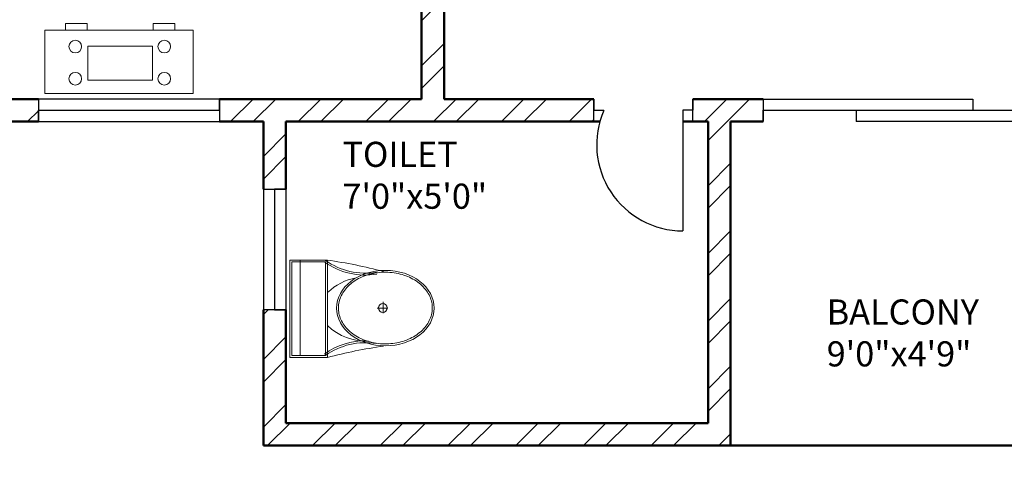
# Model space of a CAD drawing. Units: inches. Extents: x 963 to 2075, y 289 to 2657.
# Tile 45 of 98: x 1689 to 1885, y 1474 to 1563. Entities that reach past the tile are written whole.
import ezdxf

# ---------------------------------------------------------------- set-up
doc = ezdxf.new("R2010")
doc.units = ezdxf.units.IN
for name, color, linetype, lineweight in [('A-AREA-IDEN', 7, 'Continuous', 18), ('A-DOOR', 4, 'Continuous', 25), ('A-FLOR-FIXT', 9, 'Continuous', 18), ('A-GLAZ', 3, 'Continuous', 25), ('A-WALL', 7, 'Continuous', 50), ('A-WALL-PATT', 8, 'Continuous', 13)]:
    doc.layers.add(name, color=color, linetype=linetype, lineweight=lineweight)
doc.styles.get("Standard").update_dxf_attribs({"font": 'arial.ttf'})

# ---------------------------------------------------------------- blocks, each defined once
blk = doc.blocks.new('A$C31115884')
for p, q in [((283.1, 497.7), (223.4, 497.7)), ((257.5, 466.4), (257.5, 523.2)), ((0, 200), (0, 0)), ((520, 200), (0, 200)), ((10, 190), (10, 10)), ((510, 190), (10, 190)), ((510, 10), (510, 190)), ((520, 0), (520, 200)), ((510, 54.5), (0, 54.5)), ((10, 10), (510, 10)), ((0, 0), (520, 0))]:
    blk.add_line(p, q)
blk.add_circle((255.6, 496.4), 23.6)
for centre, radius, start, end in [((2777.7, -204.6), 2807, 165.4549, 171.7133), ((3237, 905), 2807, 188.2867, 194.5451), ((-294.5, 403.3), 364.7, 324.2091, 9.3499), ((-294.5, 403.3), 374.7, 324.2091, 9.3499), ((805.8, 403.3), 364.7, 170.6501, 215.7909), ((139.5, 406.2), 293.5, 315.8436, 2.6563), ((805.8, 403.3), 374.7, 179.2036, 215.7909), ((383.6, 406.2), 293.5, 190.2774, 224.1564)]:
    blk.add_arc(centre, radius, start, end)
blk.add_ellipse((256.2, 509.9), major_axis=(0, -260.7), ratio=0.772727)
blk.add_open_spline([(256.2, 259.2), (263.1, 259.2), (270, 259.7), (287.8, 262.3), (298.7, 265.1), (319.9, 273.1), (330.2, 278.4), (350.1, 291.1), (359.7, 298.7), (377.7, 315.9), (386.2, 325.5), (401.7, 346.6), (408.8, 358.1), (421.3, 382.5), (426.8, 395.5), (435.9, 422.4), (439.5, 436.4), (444.8, 465.1), (446.5, 479.7), (447.9, 509.2), (447.6, 524), (445, 553.3), (442.7, 567.8), (436.3, 596), (432.1, 609.7), (421.9, 636), (416, 648.6), (402.5, 672.1), (395, 683), (378.6, 703), (369.8, 712.1), (351.1, 728), (341.3, 734.8), (320.9, 746.2), (310.4, 750.7), (288.9, 757.3), (278, 759.4), (256, 761), (245, 760.6), (223.1, 757.2), (212.3, 754.3), (191.1, 746.1), (180.8, 740.7), (160.9, 727.8), (151.4, 720.1), (133.5, 702.7), (125.1, 693), (109.6, 671.7), (102.6, 660.2), (90.2, 635.7), (84.9, 622.7), (76, 595.6), (72.4, 581.6), (67.2, 552.9), (65.6, 538.2), (64.4, 508.8), (64.8, 494), (67.5, 464.7), (69.9, 450.2), (76.6, 422), (80.8, 408.3), (91.1, 382.2), (97.2, 369.7), (110.8, 346.3), (118.4, 335.4), (134.8, 315.6), (143.7, 306.7), (162.4, 290.9), (172.3, 284.2), (192.8, 273), (203.3, 268.6), (224.8, 262.2), (235.8, 260.2), (249.9, 259.3), (253, 259.2), (256.2, 259.2)], degree=3, knots=[0, 0, 0, 0, 0.110105, 0.110105, 0.285049, 0.285049, 0.459994, 0.459994, 0.634938, 0.634938, 0.809882, 0.809882, 0.984827, 0.984827, 1.159771, 1.159771, 1.334715, 1.334715, 1.50966, 1.50966, 1.684604, 1.684604, 1.859549, 1.859549, 2.034493, 2.034493, 2.209437, 2.209437, 2.384382, 2.384382, 2.559326, 2.559326, 2.73427, 2.73427, 2.909215, 2.909215, 3.084159, 3.084159, 3.259103, 3.259103, 3.434048, 3.434048, 3.608992, 3.608992, 3.783936, 3.783936, 3.958881, 3.958881, 4.133825, 4.133825, 4.30877, 4.30877, 4.483714, 4.483714, 4.658658, 4.658658, 4.833603, 4.833603, 5.008547, 5.008547, 5.183491, 5.183491, 5.358436, 5.358436, 5.53338, 5.53338, 5.708324, 5.708324, 5.883269, 5.883269, 6.058213, 6.058213, 6.233158, 6.233158, 6.283185, 6.283185, 6.283185, 6.283185])

msp = doc.modelspace()

# ---------------------------------------------------------------- hatches: boundary and pattern name
at = {"layer": 'A-WALL-PATT'}
h = msp.add_hatch(dxfattribs=at)
h.set_pattern_fill('ANSI32', color=256)
h.paths.add_polyline_path([(1296.92, 2558.32), (1203.92, 2558.32), (1203.92, 2493.82), (1191.53, 2493.82), (1191.53, 2489.32), (1211.06, 2489.32), (1211.06, 2492.02), (1211.06, 2493.82), (1208.42, 2493.82), (1208.42, 2553.82), (1292.42, 2553.82), (1292.42, 2538.86), (1296.92, 2538.86)])
h.paths.add_polyline_path([(1442.42, 2558.32), (1349.42, 2558.32), (1349.42, 2538.94), (1353.92, 2538.94), (1353.92, 2553.82), (1437.92, 2553.82), (1437.92, 2493.82), (1434.54, 2493.82), (1434.54, 2489.32), (1448.31, 2489.32), (1448.31, 2491.57), (1448.31, 2493.82), (1442.42, 2493.82)])
h.paths.add_polyline_path([(1415.55, 2491.57), (1415.55, 2493.82), (1340.94, 2493.82), (1340.94, 2489.32), (1371.92, 2489.32), (1371.92, 2378.32), (1367.6, 2378.32), (1367.6, 2373.82), (1371.92, 2373.82), (1371.92, 2355.19), (1376.42, 2355.19), (1376.42, 2489.32), (1415.55, 2489.32)])
h.paths.add_polyline_path([(1304.94, 2491.57), (1304.94, 2493.82), (1296.92, 2493.82), (1296.92, 2514.86), (1292.42, 2514.86), (1292.42, 2493.82), (1232.81, 2493.82), (1232.81, 2489.32), (1256.42, 2489.32), (1256.42, 2327.32), (1253.71, 2327.32), (1253.71, 2322.82), (1328.42, 2322.82), (1328.42, 2331.15), (1323.92, 2331.15), (1323.92, 2327.32), (1260.92, 2327.32), (1260.92, 2373.82), (1323.92, 2373.82), (1323.92, 2357.81), (1328.42, 2357.81), (1328.42, 2373.82), (1346.01, 2373.82), (1346.01, 2376.07), (1346.01, 2378.32), (1260.92, 2378.32), (1260.92, 2489.32), (1304.94, 2489.32)])
h.paths.add_polyline_path([(1226.65, 2327.32), (1124.42, 2327.32), (1124.42, 2347.45), (1119.92, 2347.45), (1119.92, 2322.82), (1163.42, 2322.82), (1163.42, 2305.43), (1165.67, 2305.43), (1167.92, 2305.43), (1167.92, 2322.82), (1226.65, 2322.82), (1226.65, 2325.07)])
h.paths.add_polyline_path([(1095.92, 2489.32), (1124.42, 2489.32), (1131.53, 2489.32), (1131.53, 2491.57), (1131.53, 2493.82), (1119.92, 2493.82), (1091.42, 2493.82), (1091.42, 2417.32), (1095.92, 2417.32), (1119.92, 2417.32), (1119.92, 2407.45), (1124.42, 2407.45), (1124.42, 2421.82), (1095.92, 2421.82)])
h.paths.add_polyline_path([(1512.92, 2558.32), (1508.42, 2558.32), (1508.42, 2493.82), (1503.4, 2493.82), (1503.4, 2489.32), (1508.42, 2489.32), (1508.42, 2327.32), (1376.42, 2327.32), (1376.42, 2330.27), (1371.92, 2330.27), (1371.92, 2298.74), (1376.42, 2298.74), (1376.42, 2322.82), (1508.42, 2322.82), (1508.42, 2165.32), (1504.26, 2165.32), (1504.26, 2160.82), (1508.42, 2160.82), (1508.42, 2108.32), (1512.92, 2108.32), (1512.92, 2160.82), (1516.18, 2160.82), (1516.18, 2163.07), (1516.18, 2165.32), (1512.92, 2165.32), (1512.92, 2322.82), (1644.92, 2322.82), (1644.92, 2298.74), (1649.42, 2298.74), (1649.42, 2322.82), (1649.42, 2330.94), (1647.17, 2330.94), (1644.92, 2330.94), (1644.92, 2327.32), (1512.92, 2327.32), (1512.92, 2489.32), (1516.76, 2489.32), (1516.76, 2491.57), (1516.76, 2493.82), (1512.92, 2493.82)])
h.paths.add_polyline_path([(1671.92, 2558.32), (1578.92, 2558.32), (1578.92, 2493.82), (1573.53, 2493.82), (1573.53, 2489.32), (1586.54, 2489.32), (1586.54, 2491.57), (1586.54, 2493.82), (1583.42, 2493.82), (1583.42, 2553.82), (1667.42, 2553.82), (1667.42, 2541.11), (1671.92, 2541.11)])
h.paths.add_polyline_path([(1681.26, 2493.82), (1671.92, 2493.82), (1671.92, 2517.11), (1667.42, 2517.11), (1667.42, 2493.82), (1610.22, 2493.82), (1610.22, 2489.32), (1644.92, 2489.32), (1644.92, 2357.87), (1649.42, 2357.87), (1649.42, 2373.82), (1652.2, 2373.82), (1652.2, 2375.83), (1652.2, 2378.32), (1649.42, 2378.32), (1649.42, 2489.32), (1681.26, 2489.32), (1681.26, 2491.57)])
h.paths.add_polyline_path([(1821.92, 2558.32), (1728.92, 2558.32), (1728.92, 2541), (1733.42, 2541), (1733.42, 2553.82), (1817.42, 2553.82), (1817.42, 2493.82), (1813.51, 2493.82), (1813.51, 2489.32), (1830.08, 2489.32), (1830.08, 2491.57), (1830.08, 2493.82), (1821.92, 2493.82)])
h.paths.add_polyline_path([(1794.24, 2493.82), (1717.26, 2493.82), (1717.26, 2489.32), (1760.42, 2489.32), (1760.42, 2378.32), (1674.4, 2378.32), (1674.4, 2373.82), (1692.92, 2373.82), (1692.92, 2356.95), (1697.42, 2356.95), (1697.42, 2373.82), (1760.42, 2373.82), (1760.42, 2327.32), (1697.42, 2327.32), (1697.42, 2333.34), (1692.92, 2333.34), (1692.92, 2322.82), (1768.04, 2322.82), (1768.04, 2325.07), (1768.04, 2327.32), (1764.92, 2327.32), (1764.92, 2489.32), (1794.24, 2489.32)])
h.paths.add_polyline_path([(1733.42, 2517), (1728.92, 2517), (1728.92, 2493.82), (1733.42, 2493.82)], flags=17)
h.paths.add_polyline_path([(1929.92, 2493.82), (1890.08, 2493.82), (1890.08, 2489.32), (1896.92, 2489.32), (1925.42, 2489.32), (1925.42, 2421.82), (1896.92, 2421.82), (1896.92, 2408.32), (1901.42, 2408.32), (1901.42, 2417.32), (1925.42, 2417.32), (1929.92, 2417.32)])
h.paths.add_polyline_path([(1901.42, 2348.32), (1896.92, 2348.32), (1896.92, 2327.32), (1800.42, 2327.32), (1800.42, 2322.82), (1853.42, 2322.82), (1853.42, 2309.45), (1857.92, 2309.45), (1857.92, 2322.82), (1901.42, 2322.82)])
h.paths.add_polyline_path([(1857.92, 2249.45), (1853.42, 2249.45), (1853.42, 2214.82), (1686.31, 2214.82), (1686.31, 2210.32), (1853.42, 2210.32), (1853.42, 2202.13), (1857.92, 2202.13), (1857.92, 2210.32)])
h.paths.add_polyline_path([(1857.92, 2142.13), (1853.42, 2142.13), (1853.42, 2115.42), (1841.42, 2115.42), (1841.42, 2088.53), (1841.42, 2046.95), (1845.92, 2046.95), (1845.92, 2110.92), (1905.92, 2110.92), (1905.92, 2092.52), (1910.42, 2092.52), (1910.42, 2115.42), (1857.92, 2115.42)])
h.paths.add_polyline_path([(1532.44, 1482.34), (1573.46, 1482.34), (1573.46, 1501), (1532.44, 1501)], flags=9)
h.paths.add_polyline_path([(1438.66, 1486.3), (1479.68, 1486.3), (1479.68, 1504.96), (1438.66, 1504.96)], flags=9)
h.paths.add_polyline_path([(1411.22, 1365.31), (1659.14, 1365.31), (1659.14, 1402.4), (1411.22, 1402.4)], flags=9)
h.paths.add_polyline_path([(1185.67, 2296.3), (1248.16, 2296.3), (1248.16, 2314.95), (1185.67, 2314.95)], flags=9)
h.paths.add_polyline_path([(1177.31, 2187.35), (1216.15, 2187.35), (1216.15, 2206.01), (1177.31, 2206.01)], flags=9)
h.paths.add_polyline_path([(1295.1, 1602.08), (1328.26, 1602.08), (1328.26, 1620.74), (1295.1, 1620.74)], flags=9)
h.paths.add_polyline_path([(1525.13, 2005.99), (1558.39, 2005.99), (1558.39, 2024.65), (1525.13, 2024.65)], flags=9)
h.paths.add_polyline_path([(1459.61, 1977.13), (1472.19, 1977.13), (1472.19, 1987.43), (1459.61, 1987.43)], flags=9)
h.paths.add_polyline_path([(1467.81, 2053.68), (1480.02, 2053.68), (1480.02, 2063.98), (1467.81, 2063.98)], flags=9)
h.paths.add_polyline_path([(1555.18, 2119.02), (1584.56, 2119.02), (1584.56, 2137.68), (1555.18, 2137.68)], flags=25)
h.paths.add_polyline_path([(1405.39, 2115.29), (1444.48, 2115.29), (1444.48, 2133.95), (1405.39, 2133.95)], flags=25)
h.paths.add_polyline_path([(1698.48, 2004.26), (1727.69, 2004.26), (1727.69, 2022.92), (1698.48, 2022.92)], flags=9)
h.paths.add_polyline_path([(1612.16, 1972.86), (1629.02, 1972.86), (1629.02, 1983.16), (1612.16, 1983.16)], flags=9)
h.paths.add_polyline_path([(1608.29, 2060.04), (1625.15, 2060.04), (1625.15, 2070.34), (1608.29, 2070.34)], flags=9)
h.paths.add_polyline_path([(1527.95, 1684.4), (1566.79, 1684.4), (1566.79, 1703.06), (1527.95, 1703.06)], flags=9)
h.paths.add_polyline_path([(1422.79, 1683.59), (1461.63, 1683.59), (1461.63, 1702.25), (1422.79, 1702.25)], flags=9)
h.paths.add_polyline_path([(1531.26, 1732.46), (1574.01, 1732.46), (1574.01, 1751.12), (1531.26, 1751.12)], flags=9)
h.paths.add_polyline_path([(1402.87, 1732.85), (1439.8, 1732.85), (1439.8, 1751.5), (1402.87, 1751.5)], flags=9)
h.paths.add_polyline_path([(1243.12, 1923.13), (1281.96, 1923.13), (1281.96, 1941.79), (1243.12, 1941.79)], flags=9)
h.paths.add_polyline_path([(1181.75, 1792.27), (1244.24, 1792.27), (1244.24, 1810.93), (1181.75, 1810.93)], flags=9)
h.paths.add_polyline_path([(1265.82, 1670.3), (1316.07, 1670.3), (1316.07, 1688.96), (1265.82, 1688.96)], flags=9)
h.paths.add_polyline_path([(1140.26, 1676.05), (1179.1, 1676.05), (1179.1, 1694.71), (1140.26, 1694.71)], flags=9)
h.paths.add_polyline_path([(1107.49, 1490.89), (1143.37, 1490.89), (1143.37, 1509.55), (1107.49, 1509.55)], flags=9)
h.paths.add_polyline_path([(1217.58, 1483.9), (1246.74, 1483.9), (1246.74, 1502.56), (1217.58, 1502.56)], flags=9)
h.paths.add_polyline_path([(1389.21, 1486.92), (1418.37, 1486.92), (1418.37, 1505.58), (1389.21, 1505.58)], flags=9)
h.paths.add_polyline_path([(1672.21, 1602.08), (1705.37, 1602.08), (1705.37, 1620.74), (1672.21, 1620.74)], flags=9)
h.paths.add_polyline_path([(1752.08, 1522.64), (1781.24, 1522.64), (1781.24, 1541.3), (1752.08, 1541.3)], flags=9)
h.paths.add_polyline_path([(1848.27, 1491.26), (1884.16, 1491.26), (1884.16, 1509.92), (1848.27, 1509.92)], flags=9)
h.paths.add_polyline_path([(1822.47, 1685.62), (1861.31, 1685.62), (1861.31, 1704.28), (1822.47, 1704.28)], flags=9)
h.paths.add_polyline_path([(1713.19, 1672.23), (1763.44, 1672.23), (1763.44, 1690.89), (1713.19, 1690.89)], flags=9)
h.paths.add_polyline_path([(1736.62, 1790.58), (1799.11, 1790.58), (1799.11, 1809.24), (1736.62, 1809.24)], flags=9)
h.paths.add_polyline_path([(1691.49, 1916.36), (1730.33, 1916.36), (1730.33, 1935.01), (1691.49, 1935.01)], flags=9)
h.paths.add_polyline_path([(1764.87, 1973.92), (1794.31, 1973.92), (1794.31, 1992.58), (1764.87, 1992.58)], flags=9)
h.paths.add_polyline_path([(1767.85, 2034.02), (1797.29, 2034.02), (1797.29, 2052.67), (1767.85, 2052.67)], flags=9)
h.paths.add_polyline_path([(1851.59, 2060.33), (1880.75, 2060.33), (1880.75, 2078.99), (1851.59, 2078.99)], flags=25)
h.paths.add_polyline_path([(1688.49, 2086.87), (1727.33, 2086.87), (1727.33, 2105.53), (1688.49, 2105.53)], flags=9)
h.paths.add_polyline_path([(1537.74, 2293.58), (1580.49, 2293.58), (1580.49, 2312.24), (1537.74, 2312.24)], flags=25)
h.paths.add_polyline_path([(1425.59, 2296.11), (1468.34, 2296.11), (1468.34, 2314.77), (1425.59, 2314.77)], flags=25)
h.paths.add_polyline_path([(1278.52, 2004.18), (1307.72, 2004.18), (1307.72, 2022.84), (1278.52, 2022.84)], flags=9)
h.paths.add_polyline_path([(1193.28, 1973.63), (1222.72, 1973.63), (1222.72, 1992.29), (1193.28, 1992.29)], flags=9)
h.paths.add_polyline_path([(1192.41, 2040.58), (1221.84, 2040.58), (1221.84, 2059.23), (1192.41, 2059.23)], flags=9)
h.paths.add_polyline_path([(1130.6, 1951.39), (1159.76, 1951.39), (1159.76, 1970.05), (1130.6, 1970.05)], flags=9)
h.paths.add_polyline_path([(1132.83, 2052.49), (1161.98, 2052.49), (1161.98, 2071.15), (1132.83, 2071.15)], flags=9)
h.paths.add_polyline_path([(1265.13, 2334.62), (1315.38, 2334.62), (1315.38, 2353.28), (1265.13, 2353.28)], flags=25)
h.paths.add_polyline_path([(1136.74, 2330.79), (1175.58, 2330.79), (1175.58, 2349.44), (1136.74, 2349.44)], flags=9)
h.paths.add_polyline_path([(1287.42, 2417.2), (1320.58, 2417.2), (1320.58, 2435.86), (1287.42, 2435.86)], flags=25)
h.paths.add_polyline_path([(1430.99, 2329.16), (1469.83, 2329.16), (1469.83, 2347.82), (1430.99, 2347.82)], flags=25)
h.paths.add_polyline_path([(1525.42, 2329.21), (1564.26, 2329.21), (1564.26, 2347.87), (1525.42, 2347.87)], flags=25)
h.paths.add_polyline_path([(1684.52, 2382.8), (1717.68, 2382.8), (1717.68, 2401.46), (1684.52, 2401.46)], flags=25)
h.paths.add_polyline_path([(1704.81, 2340.29), (1755.05, 2340.29), (1755.05, 2358.95), (1704.81, 2358.95)], flags=25)
h.paths.add_polyline_path([(1694.11, 2287.76), (1756.6, 2287.76), (1756.6, 2306.41), (1694.11, 2306.41)], flags=9)
h.paths.add_polyline_path([(1815.78, 2329.86), (1854.62, 2329.86), (1854.62, 2348.52), (1815.78, 2348.52)], flags=9)
h.paths.add_polyline_path([(1842.87, 2514.26), (1878.76, 2514.26), (1878.76, 2532.91), (1842.87, 2532.91)], flags=9)
h.paths.add_polyline_path([(1769.51, 2531.45), (1798.67, 2531.45), (1798.67, 2550.1), (1769.51, 2550.1)], flags=25)
h.paths.add_polyline_path([(1594.77, 2518.47), (1623.93, 2518.47), (1623.93, 2537.13), (1594.77, 2537.13)], flags=25)
h.paths.add_polyline_path([(1520.72, 2516.18), (1556.61, 2516.18), (1556.61, 2534.84), (1520.72, 2534.84)], flags=25)
h.paths.add_polyline_path([(1464.46, 2516.69), (1500.34, 2516.69), (1500.34, 2535.35), (1464.46, 2535.35)], flags=25)
h.paths.add_polyline_path([(1365.7, 2528.97), (1394.85, 2528.97), (1394.85, 2547.63), (1365.7, 2547.63)], flags=25)
h.paths.add_polyline_path([(1222.84, 2516.23), (1252, 2516.23), (1252, 2534.89), (1222.84, 2534.89)], flags=25)
h.paths.add_polyline_path([(1104.55, 2509.6), (1140.43, 2509.6), (1140.43, 2528.26), (1104.55, 2528.26)], flags=9)
h = msp.add_hatch(dxfattribs=at)
h.set_pattern_fill('ANSI32', color=256)
h.paths.add_polyline_path([(1335.97, 2212.57), (1335.97, 2214.82), (1167.92, 2214.82), (1167.92, 2245.43), (1163.42, 2245.43), (1163.42, 2210.32), (1163.42, 2194.81), (1167.92, 2194.81), (1167.92, 2210.32), (1335.97, 2210.32)])
h.paths.add_polyline_path([(1532.44, 1482.34), (1573.46, 1482.34), (1573.46, 1501), (1532.44, 1501)], flags=9)
h.paths.add_polyline_path([(1438.66, 1486.3), (1479.68, 1486.3), (1479.68, 1504.96), (1438.66, 1504.96)], flags=9)
h.paths.add_polyline_path([(1411.22, 1365.31), (1659.14, 1365.31), (1659.14, 1402.4), (1411.22, 1402.4)], flags=9)
h.paths.add_polyline_path([(1185.67, 2296.3), (1248.16, 2296.3), (1248.16, 2314.95), (1185.67, 2314.95)], flags=9)
h.paths.add_polyline_path([(1177.31, 2187.35), (1216.15, 2187.35), (1216.15, 2206.01), (1177.31, 2206.01)], flags=9)
h.paths.add_polyline_path([(1295.1, 1602.08), (1328.26, 1602.08), (1328.26, 1620.74), (1295.1, 1620.74)], flags=9)
h.paths.add_polyline_path([(1525.13, 2005.99), (1558.39, 2005.99), (1558.39, 2024.65), (1525.13, 2024.65)], flags=9)
h.paths.add_polyline_path([(1459.61, 1977.13), (1472.19, 1977.13), (1472.19, 1987.43), (1459.61, 1987.43)], flags=9)
h.paths.add_polyline_path([(1467.81, 2053.68), (1480.02, 2053.68), (1480.02, 2063.98), (1467.81, 2063.98)], flags=9)
h.paths.add_polyline_path([(1555.18, 2119.02), (1584.56, 2119.02), (1584.56, 2137.68), (1555.18, 2137.68)], flags=9)
h.paths.add_polyline_path([(1405.39, 2115.29), (1444.48, 2115.29), (1444.48, 2133.95), (1405.39, 2133.95)], flags=9)
h.paths.add_polyline_path([(1698.48, 2004.26), (1727.69, 2004.26), (1727.69, 2022.92), (1698.48, 2022.92)], flags=9)
h.paths.add_polyline_path([(1612.16, 1972.86), (1629.02, 1972.86), (1629.02, 1983.16), (1612.16, 1983.16)], flags=9)
h.paths.add_polyline_path([(1608.29, 2060.04), (1625.15, 2060.04), (1625.15, 2070.34), (1608.29, 2070.34)], flags=9)
h.paths.add_polyline_path([(1527.95, 1684.4), (1566.79, 1684.4), (1566.79, 1703.06), (1527.95, 1703.06)], flags=9)
h.paths.add_polyline_path([(1422.79, 1683.59), (1461.63, 1683.59), (1461.63, 1702.25), (1422.79, 1702.25)], flags=9)
h.paths.add_polyline_path([(1531.26, 1732.46), (1574.01, 1732.46), (1574.01, 1751.12), (1531.26, 1751.12)], flags=9)
h.paths.add_polyline_path([(1402.87, 1732.85), (1439.8, 1732.85), (1439.8, 1751.5), (1402.87, 1751.5)], flags=9)
h.paths.add_polyline_path([(1243.12, 1923.13), (1281.96, 1923.13), (1281.96, 1941.79), (1243.12, 1941.79)], flags=9)
h.paths.add_polyline_path([(1181.75, 1792.27), (1244.24, 1792.27), (1244.24, 1810.93), (1181.75, 1810.93)], flags=9)
h.paths.add_polyline_path([(1265.82, 1670.3), (1316.07, 1670.3), (1316.07, 1688.96), (1265.82, 1688.96)], flags=9)
h.paths.add_polyline_path([(1140.26, 1676.05), (1179.1, 1676.05), (1179.1, 1694.71), (1140.26, 1694.71)], flags=9)
h.paths.add_polyline_path([(1107.49, 1490.89), (1143.37, 1490.89), (1143.37, 1509.55), (1107.49, 1509.55)], flags=9)
h.paths.add_polyline_path([(1217.58, 1483.9), (1246.74, 1483.9), (1246.74, 1502.56), (1217.58, 1502.56)], flags=9)
h.paths.add_polyline_path([(1389.21, 1486.92), (1418.37, 1486.92), (1418.37, 1505.58), (1389.21, 1505.58)], flags=9)
h.paths.add_polyline_path([(1672.21, 1602.08), (1705.37, 1602.08), (1705.37, 1620.74), (1672.21, 1620.74)], flags=9)
h.paths.add_polyline_path([(1752.08, 1522.64), (1781.24, 1522.64), (1781.24, 1541.3), (1752.08, 1541.3)], flags=9)
h.paths.add_polyline_path([(1848.27, 1491.26), (1884.16, 1491.26), (1884.16, 1509.92), (1848.27, 1509.92)], flags=9)
h.paths.add_polyline_path([(1822.47, 1685.62), (1861.31, 1685.62), (1861.31, 1704.28), (1822.47, 1704.28)], flags=9)
h.paths.add_polyline_path([(1713.19, 1672.23), (1763.44, 1672.23), (1763.44, 1690.89), (1713.19, 1690.89)], flags=9)
h.paths.add_polyline_path([(1736.62, 1790.58), (1799.11, 1790.58), (1799.11, 1809.24), (1736.62, 1809.24)], flags=9)
h.paths.add_polyline_path([(1691.49, 1916.36), (1730.33, 1916.36), (1730.33, 1935.01), (1691.49, 1935.01)], flags=9)
h.paths.add_polyline_path([(1764.87, 1973.92), (1794.31, 1973.92), (1794.31, 1992.58), (1764.87, 1992.58)], flags=9)
h.paths.add_polyline_path([(1767.85, 2034.02), (1797.29, 2034.02), (1797.29, 2052.67), (1767.85, 2052.67)], flags=9)
h.paths.add_polyline_path([(1851.59, 2060.33), (1880.75, 2060.33), (1880.75, 2078.99), (1851.59, 2078.99)], flags=9)
h.paths.add_polyline_path([(1688.49, 2086.87), (1727.33, 2086.87), (1727.33, 2105.53), (1688.49, 2105.53)], flags=9)
h.paths.add_polyline_path([(1537.74, 2293.58), (1580.49, 2293.58), (1580.49, 2312.24), (1537.74, 2312.24)], flags=9)
h.paths.add_polyline_path([(1425.59, 2296.11), (1468.34, 2296.11), (1468.34, 2314.77), (1425.59, 2314.77)], flags=9)
h.paths.add_polyline_path([(1278.52, 2004.18), (1307.72, 2004.18), (1307.72, 2022.84), (1278.52, 2022.84)], flags=9)
h.paths.add_polyline_path([(1193.28, 1973.63), (1222.72, 1973.63), (1222.72, 1992.29), (1193.28, 1992.29)], flags=9)
h.paths.add_polyline_path([(1192.41, 2040.58), (1221.84, 2040.58), (1221.84, 2059.23), (1192.41, 2059.23)], flags=9)
h.paths.add_polyline_path([(1130.6, 1951.39), (1159.76, 1951.39), (1159.76, 1970.05), (1130.6, 1970.05)], flags=9)
h.paths.add_polyline_path([(1132.83, 2052.49), (1161.98, 2052.49), (1161.98, 2071.15), (1132.83, 2071.15)], flags=9)
h.paths.add_polyline_path([(1265.13, 2334.62), (1315.38, 2334.62), (1315.38, 2353.28), (1265.13, 2353.28)], flags=9)
h.paths.add_polyline_path([(1136.74, 2330.79), (1175.58, 2330.79), (1175.58, 2349.44), (1136.74, 2349.44)], flags=9)
h.paths.add_polyline_path([(1287.42, 2417.2), (1320.58, 2417.2), (1320.58, 2435.86), (1287.42, 2435.86)], flags=9)
h.paths.add_polyline_path([(1430.99, 2329.16), (1469.83, 2329.16), (1469.83, 2347.82), (1430.99, 2347.82)], flags=9)
h.paths.add_polyline_path([(1525.42, 2329.21), (1564.26, 2329.21), (1564.26, 2347.87), (1525.42, 2347.87)], flags=9)
h.paths.add_polyline_path([(1684.52, 2382.8), (1717.68, 2382.8), (1717.68, 2401.46), (1684.52, 2401.46)], flags=9)
h.paths.add_polyline_path([(1704.81, 2340.29), (1755.05, 2340.29), (1755.05, 2358.95), (1704.81, 2358.95)], flags=9)
h.paths.add_polyline_path([(1694.11, 2287.76), (1756.6, 2287.76), (1756.6, 2306.41), (1694.11, 2306.41)], flags=9)
h.paths.add_polyline_path([(1815.78, 2329.86), (1854.62, 2329.86), (1854.62, 2348.52), (1815.78, 2348.52)], flags=9)
h.paths.add_polyline_path([(1842.87, 2514.26), (1878.76, 2514.26), (1878.76, 2532.91), (1842.87, 2532.91)], flags=9)
h.paths.add_polyline_path([(1769.51, 2531.45), (1798.67, 2531.45), (1798.67, 2550.1), (1769.51, 2550.1)], flags=9)
h.paths.add_polyline_path([(1594.77, 2518.47), (1623.93, 2518.47), (1623.93, 2537.13), (1594.77, 2537.13)], flags=9)
h.paths.add_polyline_path([(1520.72, 2516.18), (1556.61, 2516.18), (1556.61, 2534.84), (1520.72, 2534.84)], flags=9)
h.paths.add_polyline_path([(1464.46, 2516.69), (1500.34, 2516.69), (1500.34, 2535.35), (1464.46, 2535.35)], flags=9)
h.paths.add_polyline_path([(1365.7, 2528.97), (1394.85, 2528.97), (1394.85, 2547.63), (1365.7, 2547.63)], flags=9)
h.paths.add_polyline_path([(1222.84, 2516.23), (1252, 2516.23), (1252, 2534.89), (1222.84, 2534.89)], flags=9)
h.paths.add_polyline_path([(1104.55, 2509.6), (1140.43, 2509.6), (1140.43, 2528.26), (1104.55, 2528.26)], flags=9)
h = msp.add_hatch(dxfattribs=at)
h.set_pattern_fill('ANSI32', color=256)
h.paths.add_polyline_path([(1910.42, 1929.42), (1910.42, 1963.51), (1905.92, 1963.51), (1905.92, 1929.42), (1845.92, 1929.42), (1845.92, 1993.37), (1843.67, 1993.37), (1841.42, 1993.37), (1841.42, 1951.16), (1841.42, 1924.92), (1853.42, 1924.92), (1853.42, 1913.07), (1857.92, 1913.07), (1857.92, 1924.92), (1910.42, 1924.92)])
h.paths.add_polyline_path([(1857.92, 1853.07), (1853.42, 1853.07), (1853.42, 1826.32), (1841.42, 1826.32), (1674.48, 1826.32), (1674.48, 1821.82), (1853.42, 1821.82), (1857.92, 1821.82)])
h.paths.add_polyline_path([(1857.92, 1821.82), (1853.42, 1821.82), (1853.42, 1807.79), (1857.92, 1807.79)])
h.paths.add_polyline_path([(1857.92, 1747.79), (1853.42, 1747.79), (1853.42, 1713.82), (1809.34, 1713.82), (1809.34, 1709.32), (1905.92, 1709.32), (1905.92, 1688.32), (1910.42, 1688.32), (1910.42, 1713.82), (1857.92, 1713.82)])
h.paths.add_polyline_path([(1830.92, 1542.82), (1837.43, 1542.82), (1837.43, 1545.07), (1837.43, 1547.32), (1823.42, 1547.32), (1823.42, 1545.07), (1823.42, 1542.82), (1826.42, 1542.82), (1826.42, 1482.82), (1742.42, 1482.82), (1742.42, 1505.39), (1737.92, 1505.39), (1737.92, 1478.32), (1830.92, 1478.32)])
h.paths.add_polyline_path([(1938.92, 1619.32), (1934.42, 1619.32), (1910.42, 1619.32), (1910.42, 1628.32), (1908.17, 1628.32), (1905.92, 1628.32), (1905.92, 1614.82), (1934.42, 1614.82), (1934.42, 1547.32), (1905.92, 1547.32), (1899.59, 1547.32), (1899.59, 1542.82), (1910.42, 1542.82), (1938.92, 1542.82)])
h.paths.add_polyline_path([(1803.68, 1547.32), (1773.92, 1547.32), (1773.92, 1709.32), (1777.76, 1709.32), (1777.76, 1713.82), (1701.92, 1713.82), (1701.92, 1697.8), (1706.42, 1697.8), (1706.42, 1709.32), (1769.42, 1709.32), (1769.42, 1662.82), (1706.42, 1662.82), (1706.42, 1674.38), (1701.92, 1674.38), (1701.92, 1662.82), (1675.67, 1662.82), (1675.67, 1658.32), (1769.42, 1658.32), (1769.42, 1547.32), (1729.17, 1547.32), (1729.17, 1542.82), (1737.92, 1542.82), (1737.92, 1529.39), (1742.42, 1529.39), (1742.42, 1542.82), (1803.68, 1542.82)])
h.paths.add_polyline_path([(1595.42, 1542.82), (1599.24, 1542.82), (1599.24, 1547.32), (1584.36, 1547.32), (1584.36, 1542.82), (1590.92, 1542.82), (1590.92, 1436.32), (1595.42, 1436.32), (1595.42, 1440.82)])
h.paths.add_polyline_path([(1693.17, 1547.32), (1649.42, 1547.32), (1649.42, 1658.32), (1652.1, 1658.32), (1652.1, 1660.57), (1652.1, 1662.82), (1649.42, 1662.82), (1649.42, 1680.94), (1647.17, 1680.94), (1644.92, 1680.94), (1644.92, 1547.32), (1622.42, 1547.32), (1622.42, 1545.07), (1622.42, 1542.82), (1649.42, 1542.82), (1679.42, 1542.82), (1679.42, 1529.85), (1681.67, 1529.85), (1683.92, 1529.85), (1683.92, 1542.82), (1693.17, 1542.82), (1693.17, 1545.07)])
h.paths.add_polyline_path([(1683.92, 1505.85), (1679.42, 1505.85), (1679.42, 1483.8), (1595.42, 1483.8), (1595.42, 1479.3), (1683.92, 1479.3)])
h.paths.add_polyline_path([(1402.99, 1547.32), (1376.42, 1547.32), (1376.42, 1675.89), (1374.17, 1675.89), (1371.92, 1675.89), (1371.92, 1662.82), (1368.88, 1662.82), (1368.88, 1658.32), (1371.92, 1658.32), (1371.92, 1547.32), (1335.46, 1547.32), (1335.46, 1542.82), (1337.42, 1542.82), (1337.42, 1526.73), (1341.92, 1526.73), (1341.92, 1542.82), (1371.92, 1542.82), (1402.99, 1542.82)])

# ---------------------------------------------------------------- linework, layer by layer
at = {"layer": 'A-DOOR'}
for p, q in [((1803.68, 1542.82), (1803.68, 1547.32)), ((1803.68, 1547.32), (1803.68, 1545.07)), ((1823.42, 1542.82), (1823.42, 1547.32)), ((1823.42, 1547.32), (1823.42, 1545.07)), ((1803.68, 1545.07), (1805.68, 1545.07)), ((1823.42, 1545.07), (1821.42, 1545.07)), ((1821.42, 1545.07), (1821.42, 1521.07))]:
    msp.add_line(p, q, dxfattribs=at)
msp.add_arc((1821.42, 1538.23), 17.16, 156.5283, 270, dxfattribs=at)
at = {"layer": 'A-FLOR-FIXT'}
for points in [[(1698.53, 1561.01), (1702.86, 1561.01), (1702.86, 1562.36), (1698.53, 1562.36)], [(1715.99, 1561.01), (1720.31, 1561.01), (1720.31, 1562.36), (1715.99, 1562.36)], [(1694.4, 1561.01), (1723.93, 1561.01), (1723.93, 1548.45), (1694.4, 1548.45)], [(1702.97, 1557.86), (1715.87, 1557.86), (1715.87, 1551.1), (1702.97, 1551.1)]]:
    msp.add_lwpolyline(points, close=True, dxfattribs=at)
for centre in [(1700.49, 1557.77), (1718.19, 1557.77), (1700.49, 1551.35), (1718.19, 1551.35)]:
    msp.add_circle(centre, 1.26, dxfattribs=at)
at = {"layer": 'A-GLAZ'}
for p, q in [((1693.17, 1547.32), (1693.17, 1542.82)), ((1729.17, 1547.32), (1693.17, 1547.32)), ((1729.17, 1545.07), (1729.17, 1547.32)), ((1729.17, 1547.32), (1729.17, 1542.82)), ((1837.43, 1547.32), (1837.43, 1542.82)), ((1837.43, 1547.32), (1879.16, 1547.32)), ((1879.16, 1547.32), (1879.16, 1545.07)), ((1693.17, 1542.82), (1693.17, 1545.07)), ((1693.17, 1545.07), (1729.17, 1545.07)), ((1837.43, 1542.82), (1837.43, 1545.07)), ((1837.43, 1545.07), (1899.59, 1545.07)), ((1855.9, 1545.07), (1855.9, 1542.82)), ((1693.17, 1542.82), (1729.17, 1542.82)), ((1899.59, 1542.82), (1855.9, 1542.82)), ((1737.92, 1529.39), (1742.42, 1529.39)), ((1737.92, 1529.39), (1737.92, 1505.39)), ((1742.42, 1529.39), (1740.17, 1529.39)), ((1740.17, 1529.39), (1740.17, 1505.39)), ((1742.42, 1529.39), (1742.42, 1505.39)), ((1742.42, 1505.39), (1737.92, 1505.39)), ((1740.17, 1505.39), (1742.42, 1505.39))]:
    msp.add_line(p, q, dxfattribs=at)
at = {"layer": 'A-WALL'}
for p, q in [((1773.92, 1709.32), (1773.92, 1547.32)), ((1769.42, 1658.32), (1769.42, 1547.32)), ((1693.17, 1547.32), (1649.42, 1547.32)), ((1769.42, 1547.32), (1729.17, 1547.32)), ((1803.68, 1547.32), (1773.92, 1547.32)), ((1837.43, 1547.32), (1823.42, 1547.32)), ((1693.17, 1542.82), (1683.92, 1542.82)), ((1737.92, 1542.82), (1729.17, 1542.82)), ((1737.92, 1542.82), (1737.92, 1529.39)), ((1742.42, 1542.82), (1742.42, 1529.39)), ((1804.88, 1542.82), (1742.42, 1542.82)), ((1826.42, 1542.82), (1821.42, 1542.82)), ((1826.42, 1542.82), (1826.42, 1482.82)), ((1830.92, 1478.32), (1830.92, 1542.82)), ((1837.43, 1542.82), (1830.92, 1542.82)), ((1737.92, 1505.39), (1737.92, 1478.32)), ((1742.42, 1505.39), (1742.42, 1482.82)), ((1826.42, 1482.82), (1742.42, 1482.82)), ((1737.92, 1478.32), (1938.92, 1478.32))]:
    msp.add_line(p, q, dxfattribs=at)

# ---------------------------------------------------------------- block references
at = {"layer": 'A-FLOR-FIXT', "xscale": 0.0372717239612423, "yscale": 0.0372717239612423, "zscale": 0.0372717239612423, "rotation": 270}
msp.add_blockref('A$C31115884', (1743.2, 1515.26), dxfattribs=at)

# ---------------------------------------------------------------- texts
at = {"layer": 'A-AREA-IDEN', "char_height": 5, "attachment_point": 1}
for s, width, insert in [('TOILET\\P7\'0"x5\'0"', 142.7344, (1753.66, 1538.81)), ('BALCONY\\P9\'0"x4\'9"', 155.8873, (1850.04, 1507.43))]:
    msp.add_mtext_dynamic_manual_height_columns(s, width=width, gutter_width=12.5, heights=[0], dxfattribs=dict(at, insert=insert))

doc.saveas('drawing.dxf')
